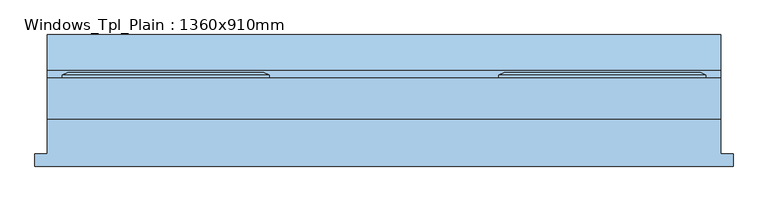
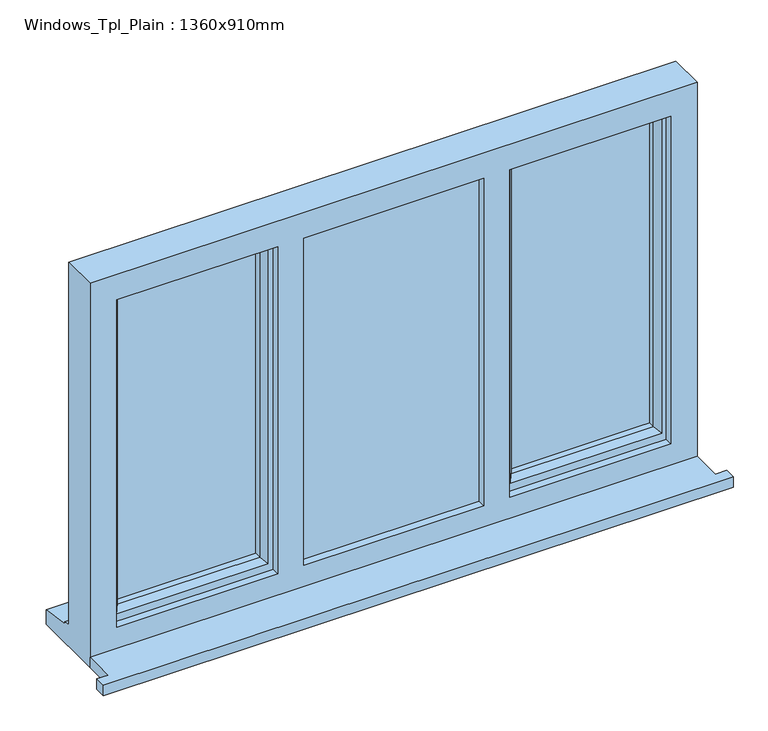
"""IFC4 building model written with IfcOpenShell, lengths in millimetres: window geometry, Windows_Tpl_Plain : 1360x910mm."""

from ifc_helpers import new_model, si_unit, frame, origin, place, context, project, spatial, polyline, outline, extrude, faceted_brep, source, transform, mapped, element, save


def windows_tpl_plain_1360x910mm_84993ef1(model_context):
    return source(origin(), model_context, "Body", "SolidModel", [
        extrude(outline(polyline([(-1206.6666667, -118.1434322), (-1206.6666667, -93.1434322), (-1181.6666667, -93.1434322), (-1181.6666667, -22.9434322), (178.3333333, -22.9434322), (178.3333333, -93.1434322), (203.3333333, -93.1434322), (203.3333333, -118.1434322), (-1206.6666667, -118.1434322)])), frame((0.0, 0.0, 1200.0), z_axis=(0.0, 0.0, 1.0), x_axis=(1.0, 0.0, 0.0)), (0.0, 0.0, 1.0), 25.0),
        faceted_brep([(-270.0, 60.0565678, 2080.0), (-270.0, 65.8300705, 2080.0), (-270.0, 65.8300705, 1253.0), (-270.0, 60.0565678, 1253.0), (-260.0, -4.9434322, 2070.0), (-260.0, 60.0565678, 2070.0), (-260.0, 60.0565678, 1263.0), (-260.0, -4.9434322, 1263.0), (-220.0, 9.5494677, 2030.0), (-230.1480377, -4.9434322, 2040.1480377), (-230.1480377, -4.9434322, 1292.8519623), (-220.0, 9.5494677, 1303.0), (-220.0, 24.0565678, 2030.0), (-220.0, 24.0565678, 1303.0), (-230.0, 48.0565678, 2040.0), (-230.0, 24.0565678, 2040.0), (-230.0, 24.0565678, 1293.0), (-230.0, 48.0565678, 1293.0), (-220.0, 65.8300705, 2030.0), (-220.0, 48.0565678, 2030.0), (-220.0, 48.0565678, 1303.0), (-220.0, 65.8300705, 1303.0), (-237.4457548, 71.6035732, 2047.4457548), (-237.4457548, 71.6035732, 1285.5542452), (-259.2153903, 71.6035732, 2069.2153903), (-259.2153903, 71.6035732, 1263.7846097), (148.3333333, 65.8300705, 1253.0), (148.3333333, 60.0565678, 1253.0), (138.3333333, 60.0565678, 1263.0), (138.3333333, -4.9434322, 1263.0), (108.4813711, -4.9434322, 1292.8519623), (98.3333333, 9.5494677, 1303.0), (98.3333333, 24.0565678, 1303.0), (108.3333333, 24.0565678, 1293.0), (108.3333333, 48.0565678, 1293.0), (98.3333333, 48.0565678, 1303.0), (98.3333333, 65.8300705, 1303.0), (115.7790881, 71.6035732, 1285.5542452), (137.5487236, 71.6035732, 1263.7846097), (148.3333333, 65.8300705, 2080.0), (148.3333333, 60.0565678, 2080.0), (138.3333333, 60.0565678, 2070.0), (138.3333333, -4.9434322, 2070.0), (108.4813711, -4.9434322, 2040.1480377), (98.3333333, 9.5494677, 2030.0), (98.3333333, 24.0565678, 2030.0), (108.3333333, 24.0565678, 2040.0), (108.3333333, 48.0565678, 2040.0), (98.3333333, 48.0565678, 2030.0), (98.3333333, 65.8300705, 2030.0), (115.7790881, 71.6035732, 2047.4457548), (137.5487236, 71.6035732, 2069.2153903)], [[[0, 1, 2, 3]], [[4, 5, 6, 7]], [[8, 9, 10, 11]], [[12, 8, 11, 13]], [[14, 15, 16, 17]], [[18, 19, 20, 21]], [[22, 18, 21, 23]], [[1, 24, 25, 2]], [[3, 2, 26, 27]], [[7, 6, 28, 29]], [[11, 10, 30, 31]], [[13, 11, 31, 32]], [[17, 16, 33, 34]], [[21, 20, 35, 36]], [[23, 21, 36, 37]], [[2, 25, 38, 26]], [[27, 26, 39, 40]], [[29, 28, 41, 42]], [[31, 30, 43, 44]], [[32, 31, 44, 45]], [[34, 33, 46, 47]], [[36, 35, 48, 49]], [[37, 36, 49, 50]], [[26, 38, 51, 39]], [[40, 39, 1, 0]], [[3, 27, 40, 0], [5, 41, 28, 6]], [[42, 41, 5, 4]], [[7, 29, 42, 4], [9, 43, 30, 10]], [[44, 43, 9, 8]], [[45, 44, 8, 12]], [[15, 46, 33, 16], [13, 32, 45, 12]], [[47, 46, 15, 14]], [[17, 34, 47, 14], [19, 48, 35, 20]], [[49, 48, 19, 18]], [[50, 49, 18, 22]], [[24, 51, 38, 25], [23, 37, 50, 22]], [[39, 51, 24, 1]]]),
        faceted_brep([(-733.3333333, 60.0565678, 2080.0), (-733.3333333, 65.8300705, 2080.0), (-1151.6666667, 65.8300705, 2080.0), (-1151.6666667, 60.0565678, 2080.0), (-743.3333333, -4.9434322, 2070.0), (-743.3333333, 60.0565678, 2070.0), (-1141.6666667, 60.0565678, 2070.0), (-1141.6666667, -4.9434322, 2070.0), (-783.3333333, 9.5494677, 2030.0), (-773.1852956, -4.9434322, 2040.1480377), (-1111.8147044, -4.9434322, 2040.1480377), (-1101.6666667, 9.5494677, 2030.0), (-783.3333333, 24.0565678, 2030.0), (-1101.6666667, 24.0565678, 2030.0), (-773.3333333, 48.0565678, 2040.0), (-773.3333333, 24.0565678, 2040.0), (-1111.6666667, 24.0565678, 2040.0), (-1111.6666667, 48.0565678, 2040.0), (-783.3333333, 65.8300705, 2030.0), (-783.3333333, 48.0565678, 2030.0), (-1101.6666667, 48.0565678, 2030.0), (-1101.6666667, 65.8300705, 2030.0), (-764.5187677, 71.6035732, 2048.8145656), (-1120.4812323, 71.6035732, 2048.8145656), (-744.964114, 71.6035732, 2068.3692194), (-1140.035886, 71.6035732, 2068.3692194), (-1151.6666667, 65.8300705, 1253.0), (-1151.6666667, 60.0565678, 1253.0), (-1141.6666667, 60.0565678, 1263.0), (-1141.6666667, -4.9434322, 1263.0), (-1111.8147044, -4.9434322, 1292.8519623), (-1101.6666667, 9.5494677, 1303.0), (-1101.6666667, 24.0565678, 1303.0), (-1111.6666667, 24.0565678, 1293.0), (-1111.6666667, 48.0565678, 1293.0), (-1101.6666667, 48.0565678, 1303.0), (-1101.6666667, 65.8300705, 1303.0), (-1120.4812323, 71.6035732, 1284.1854344), (-1140.035886, 71.6035732, 1264.6307806), (-733.3333333, 65.8300705, 1253.0), (-733.3333333, 60.0565678, 1253.0), (-743.3333333, 60.0565678, 1263.0), (-743.3333333, -4.9434322, 1263.0), (-773.1852956, -4.9434322, 1292.8519623), (-783.3333333, 9.5494677, 1303.0), (-783.3333333, 24.0565678, 1303.0), (-773.3333333, 24.0565678, 1293.0), (-773.3333333, 48.0565678, 1293.0), (-783.3333333, 48.0565678, 1303.0), (-783.3333333, 65.8300705, 1303.0), (-764.5187677, 71.6035732, 1284.1854344), (-744.964114, 71.6035732, 1264.6307806)], [[[0, 1, 2, 3]], [[4, 5, 6, 7]], [[8, 9, 10, 11]], [[12, 8, 11, 13]], [[14, 15, 16, 17]], [[18, 19, 20, 21]], [[22, 18, 21, 23]], [[1, 24, 25, 2]], [[3, 2, 26, 27]], [[7, 6, 28, 29]], [[11, 10, 30, 31]], [[13, 11, 31, 32]], [[17, 16, 33, 34]], [[21, 20, 35, 36]], [[23, 21, 36, 37]], [[2, 25, 38, 26]], [[27, 26, 39, 40]], [[0, 3, 27, 40], [41, 28, 6, 5]], [[29, 28, 41, 42]], [[4, 7, 29, 42], [43, 30, 10, 9]], [[31, 30, 43, 44]], [[32, 31, 44, 45]], [[46, 33, 16, 15], [12, 13, 32, 45]], [[34, 33, 46, 47]], [[14, 17, 34, 47], [48, 35, 20, 19]], [[36, 35, 48, 49]], [[37, 36, 49, 50]], [[51, 38, 25, 24], [22, 23, 37, 50]], [[26, 38, 51, 39]], [[40, 39, 1, 0]], [[42, 41, 5, 4]], [[44, 43, 9, 8]], [[45, 44, 8, 12]], [[47, 46, 15, 14]], [[49, 48, 19, 18]], [[50, 49, 18, 22]], [[39, 51, 24, 1]]]),
        faceted_brep([(178.3333333, -22.9434322, 2110.0), (-1181.6666667, -22.9434322, 2110.0), (-1181.6666667, -22.9434322, 1200.0), (178.3333333, -22.9434322, 1200.0), (118.3333333, -22.9434322, 2050.0), (118.3333333, -22.9434322, 1275.0), (-242.0, -22.9434322, 1275.0), (-242.0, -22.9434322, 2050.0), (-300.0, -22.9434322, 2050.0), (-300.0, -22.9434322, 1275.0), (-703.3333333, -22.9434322, 1275.0), (-703.3333333, -22.9434322, 2050.0), (-761.3333333, -22.9434322, 2050.0), (-761.3333333, -22.9434322, 1275.0), (-1121.6666667, -22.9434322, 1275.0), (-1121.6666667, -22.9434322, 2050.0), (-1181.6666667, 60.0565678, 2110.0), (-1181.6666667, 60.0565678, 1251.0), (-1181.6666667, 75.0565678, 1249.68767), (-1181.6666667, 75.0565678, 1244.7449676), (-1181.6666667, 147.5565678, 1233.8088847), (-1181.6666667, 147.5565678, 1200.0), (178.3333333, 60.0565678, 2110.0), (178.3333333, 60.0565678, 1251.0), (-1141.6666667, 60.0565678, 2070.0), (-1141.6666667, 60.0565678, 1263.0), (-743.3333333, 60.0565678, 1263.0), (-743.3333333, 60.0565678, 2070.0), (-703.3333333, 60.0565678, 2070.0), (-703.3333333, 60.0565678, 1263.0), (-300.0, 60.0565678, 1263.0), (-300.0, 60.0565678, 2070.0), (-260.0, 60.0565678, 2070.0), (-260.0, 60.0565678, 1263.0), (138.3333333, 60.0565678, 1263.0), (138.3333333, 60.0565678, 2070.0), (-1141.6666667, -4.9434322, 2070.0), (-1141.6666667, -4.9434322, 1263.0), (-713.3333333, -4.9434322, 2070.0), (-290.0, -4.9434322, 2070.0), (-290.0, -4.9434322, 1263.0), (-713.3333333, -4.9434322, 1263.0), (-300.0, -4.9434322, 2050.0), (-703.3333333, -4.9434322, 2050.0), (-703.3333333, -4.9434322, 1275.0), (-300.0, -4.9434322, 1275.0), (-260.0, -4.9434322, 2070.0), (138.3333333, -4.9434322, 2070.0), (138.3333333, -4.9434322, 1263.0), (-260.0, -4.9434322, 1263.0), (118.3333333, -4.9434322, 2050.0), (-242.0, -4.9434322, 2050.0), (-242.0, -4.9434322, 1275.0), (118.3333333, -4.9434322, 1275.0), (-743.3333333, -4.9434322, 2070.0), (-743.3333333, -4.9434322, 1263.0), (-761.3333333, -4.9434322, 2050.0), (-1121.6666667, -4.9434322, 2050.0), (-1121.6666667, -4.9434322, 1275.0), (-761.3333333, -4.9434322, 1275.0), (-703.3333333, 19.0565678, 2070.0), (-300.0, 19.0565678, 2070.0), (-290.0, 19.0565678, 2070.0), (-713.3333333, 19.0565678, 2070.0), (178.3333333, 147.5565678, 1200.0), (178.3333333, 147.5565678, 1233.8088847), (178.3333333, 75.0565678, 1244.7449676), (178.3333333, 75.0565678, 1249.68767), (-703.3333333, 19.0565678, 1263.0), (-713.3333333, 19.0565678, 1263.0), (-290.0, 19.0565678, 1263.0), (-300.0, 19.0565678, 1263.0)], [[[0, 1, 2, 3], [4, 5, 6, 7], [8, 9, 10, 11], [12, 13, 14, 15]], [[2, 1, 16, 17, 18, 19, 20, 21]], [[17, 16, 22, 23], [24, 25, 26, 27], [28, 29, 30, 31], [32, 33, 34, 35]], [[25, 24, 36, 37]], [[38, 39, 40, 41], [42, 43, 44, 45]], [[46, 47, 48, 49], [50, 51, 52, 53]], [[36, 54, 55, 37], [56, 57, 58, 59]], [[57, 15, 14, 58]], [[1, 0, 22, 16]], [[36, 24, 27, 54]], [[35, 47, 46, 32]], [[60, 28, 31, 61, 62, 39, 38, 63]], [[15, 57, 56, 12]], [[50, 4, 7, 51]], [[11, 43, 42, 8]], [[23, 22, 0, 3, 64, 65, 66, 67]], [[35, 34, 48, 47]], [[4, 50, 53, 5]], [[43, 11, 10, 44]], [[12, 56, 59, 13]], [[27, 26, 55, 54]], [[29, 28, 60, 68]], [[68, 60, 63, 69]], [[69, 63, 38, 41]], [[62, 70, 40, 39]], [[70, 62, 61, 71]], [[71, 61, 31, 30]], [[33, 32, 46, 49]], [[51, 7, 6, 52]], [[8, 42, 45, 9]], [[64, 3, 2, 21]], [[65, 64, 21, 20]], [[66, 65, 20, 19]], [[67, 66, 19, 18]], [[23, 67, 18, 17]], [[26, 25, 37, 55]], [[34, 33, 49, 48]], [[41, 40, 70, 71, 30, 29, 68, 69]], [[6, 5, 53, 52]], [[45, 44, 10, 9]], [[59, 58, 14, 13]]]),
        extrude(outline(polyline([(-773.3333333, 24.0565678), (-1111.6666667, 24.0565678), (-1111.6666667, 48.0565678), (-773.3333333, 48.0565678), (-773.3333333, 24.0565678)])), frame((0.0, 0.0, 1293.0), z_axis=(0.0, 0.0, 1.0), x_axis=(1.0, 0.0, 0.0)), (0.0, 0.0, 1.0), 747.0),
        extrude(outline(polyline([(-713.3333333, 19.0565678), (-290.0, 19.0565678), (-290.0, -4.9434322), (-713.3333333, -4.9434322), (-713.3333333, 19.0565678)])), frame((0.0, 0.0, 1263.0), z_axis=(0.0, 0.0, 1.0), x_axis=(1.0, 0.0, 0.0)), (0.0, 0.0, 1.0), 807.0),
        extrude(outline(polyline([(108.3333333, 24.0565678), (-230.0, 24.0565678), (-230.0, 48.0565678), (108.3333333, 48.0565678), (108.3333333, 24.0565678)])), frame((0.0, 0.0, 1293.0), z_axis=(0.0, 0.0, 1.0), x_axis=(1.0, 0.0, 0.0)), (0.0, 0.0, 1.0), 747.0),
    ])


if __name__ == "__main__":
    model = new_model("IFC4")
    model_context = context("Model", 3, world=origin())
    ifc_project = project(units=[si_unit("LENGTHUNIT", "METRE", prefix="MILLI")], contexts=[model_context])
    site = spatial("IfcSite", under=ifc_project)
    building = spatial("IfcBuilding", under=site)
    placement = place(None, origin())
    windows_tpl_plain_1360x910mm_shape = windows_tpl_plain_1360x910mm_84993ef1(model_context)
    element("IfcWindow", 1, ObjectType="Windows_Tpl_Plain : 1360x910mm", at=placement, inside=building, context=model_context, shape_type="MappedRepresentation", body=[
        mapped(windows_tpl_plain_1360x910mm_shape, transform((0.0, 0.0, 0.0), x_axis=(1.0, 0.0, 0.0), y_axis=(0.0, 1.0, 0.0), z_axis=(0.0, 0.0, 1.0))),
    ])
    save(model, "model.ifc")

# Revit data of these elements
# Type "Windows_Tpl_Plain : 1360x910mm"
#   Type Mark = "20"
#   Operation = "TriplePanelVertical"
#   Construction Type Id = "GSP4R"
#   Manufacturer = "Revit"
#   Keynote = "L10"
#   Analytic Construction = "1/8 in Pilkington single glazing"
#   Wrap Layers (Ext) from Ext = 0' - 4.03543"
#   Wrap Layers (Int) from Ext = 0' - 6.98819"
#   Window Board Projection = 0' - 0.98425"
#   Window Board Extension = 0' - 0.98425"
#   Visual Light Transmittance = 0.9
#   Solar Heat Gain Coefficient = 0.78
#   Rough Width = 4' - 5.54331"
#   Rough Height = 2' - 11.82677"
#   Height = 2' - 11.82677"
#   Width = 4' - 5.54331"
#   Heat Transfer Coefficient (U) = 0.6496 BTU/(h·ft²·°F)
#   Glazing Thickness = 0' - 0.94488"
#   FrameOffset - External = 0' - 1.9685"
#   Frame Depth = 0' - 2.55906"
#   Default Head Height = 6' - 11.07087"
#   Cill Depth = 0' - 3.44488"
#   Cavity Closer Width = 0' - 1.9685"
#   Cavity Closer Offset from Ext = 0' - 4.03543"
#   Cavity Closer Depth = 0' - 3.34646"
#   Vis - Cavity Closers = yes
#   Define Thermal Properties by = 1
#   Material Trim = Window Frame
#   Material Glass = Glass
#   Material Frame = Window Frame
#   Wall Closure = (empty or 0)
# Element 1 (IfcWindow, "Windows_Tpl_Plain : 1360x910mm")
#   Materials on its faces: "Window Frame", "Glass"
# Materials
#   "Window Frame": colour RGB 249 249 249, transparency 0
#   "Glass": class "Glass", colour RGB 0 128 192, transparency 0.75, Description = "Soda Lime Glass", Cost = 0
